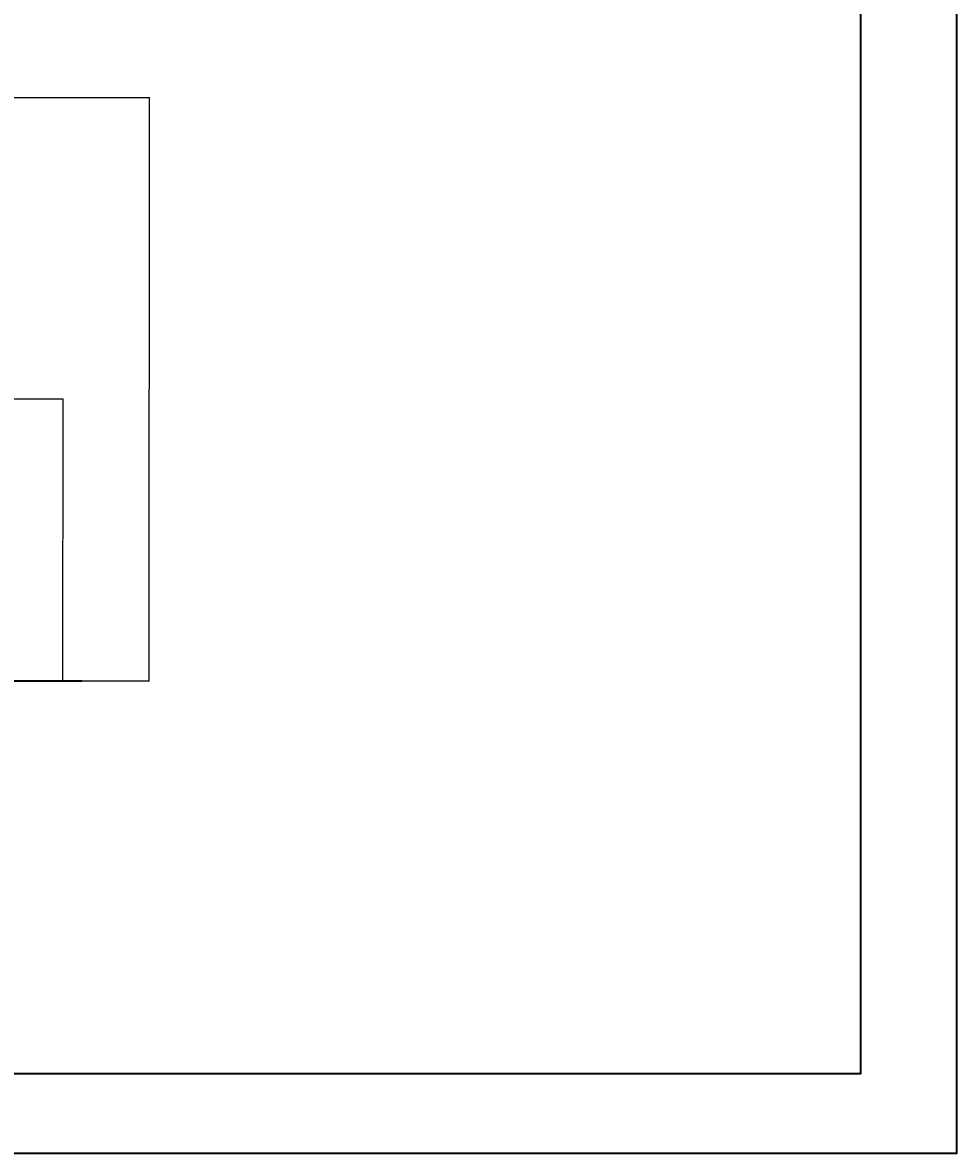
# Model space of a CAD drawing. Units: inches. Extents: x -934 to 898, y -1502 to 444.
# Tile 4 of 10: x 268 to 898, y -1502 to -739. Entities that reach past the tile are written whole.
import ezdxf

# ---------------------------------------------------------------- set-up
doc = ezdxf.new("R2010")
doc.units = ezdxf.units.IN
doc.header["$MEASUREMENT"] = 0
for name, color, linetype, lineweight in [('A-ANNO-DIMS', 2, 'Continuous', 18), ('A-ANNO-TTLB', 7, 'Continuous', 35), ('L-GRND', 7, 'Continuous', 35)]:
    doc.layers.add(name, color=color, linetype=linetype, lineweight=lineweight)
doc.styles.get("Standard").update_dxf_attribs({"font": 'arial.ttf'})
doc.dimstyles.get("Standard").update_dxf_attribs({"dimtxt": 0.18, "dimasz": 0.18, "dimexe": 0.18, "dimexo": 0.0625, "dimgap": 0.09, "dimtad": 0, "dimtih": 1, "dimtoh": 1, "dimdec": 4, "dimzin": 0, "dimdsep": 46, "dimtxsty": 'Standard', "dimcen": 0.09, "dimadec": 0, "dimazin": 0, "dimtfac": 1, "dimtdec": 4, "dimtofl": 0, "dimtmove": 0, "dimatfit": 3, "dimfxl": 1, "dimtolj": 1, "dimtzin": 0, "dimarcsym": 0})

# ---------------------------------------------------------------- blocks, each defined once
blk = doc.blocks.new('*D108')
at = {"layer": 'A-ANNO-DIMS', "color": 0, "lineweight": -2, "transparency": 16777216}
for p, q in [((24.87, -789.83), (353.87, -789.83)), ((353.69, -790.01), (353.69, -986.24)), ((353.69, -1182.83), (353.69, -986.6)), ((250.04, -1183.01), (353.87, -1183.01))]:
    blk.add_line(p, q, dxfattribs=at)
at = {"layer": 'A-ANNO-DIMS', "color": 0, "transparency": 16777216}
for points in [[(353.66, -790.01), (353.72, -790.01), (353.69, -789.83)], [(353.66, -1182.83), (353.72, -1182.83), (353.69, -1183.01)]]:
    blk.add_solid(points, dxfattribs=at)
at = {"layer": 'Defpoints', "color": 0, "transparency": 16777216}
for p in [(24.8, -789.83), (353.69, -789.83), (249.98, -1183.01)]:
    blk.add_point(p, dxfattribs=at)
at = {"layer": 'A-ANNO-DIMS', "color": 0, "transparency": 16777216, "insert": (353.69, -986.42), "char_height": 0.18, "attachment_point": 5}
blk.add_mtext('\\A1;393.2', dxfattribs=at)
blk = doc.blocks.new('*D113')
at = {"layer": 'A-ANNO-DIMS', "color": 0, "lineweight": -2, "transparency": 16777216}
for p, q in [((250.04, -993.04), (295.66, -993.04)), ((295.48, -993.22), (295.48, -1087.84)), ((295.48, -1182.83), (295.48, -1088.21)), ((250.04, -1183.01), (295.66, -1183.01))]:
    blk.add_line(p, q, dxfattribs=at)
at = {"layer": 'A-ANNO-DIMS', "color": 0, "transparency": 16777216}
for points in [[(295.45, -993.22), (295.51, -993.22), (295.48, -993.04)], [(295.45, -1182.83), (295.51, -1182.83), (295.48, -1183.01)]]:
    blk.add_solid(points, dxfattribs=at)
at = {"layer": 'Defpoints', "color": 0, "transparency": 16777216}
for p in [(249.98, -993.04), (249.98, -1183.01), (295.48, -1183.01)]:
    blk.add_point(p, dxfattribs=at)
at = {"layer": 'A-ANNO-DIMS', "color": 0, "transparency": 16777216, "insert": (295.48, -1088.02), "char_height": 0.18, "attachment_point": 5}
blk.add_mtext('\\A1;189.97', dxfattribs=at)

msp = doc.modelspace()

# ---------------------------------------------------------------- linework, layer by layer
at = {"layer": 'A-ANNO-TTLB'}
for points in [[(-933.5092, 444.4646), (897.7239, 444.4646), (897.7239, -1501.5858), (-933.5092, -1501.5858)], [(-892.081, 380.0228), (832.9871, 380.0228), (832.9871, -1448.0237), (-892.081, -1448.0237)]]:
    msp.add_lwpolyline(points, close=True, dxfattribs=at)
at = {"layer": 'L-GRND'}
msp.add_line((-288.9776, -1183.0104), (308.1933, -1183.0104), dxfattribs=at)

# ---------------------------------------------------------------- dimensions: what is measured, and where the dimension line sits
at = {"layer": 'A-ANNO-DIMS'}
for base, p1, p2, angle, override, picture, middle in [((353.6933, -789.826), (249.977, -1183.0104), (24.8027, -789.826), 90, {"dimdec": 1, "dimlfac": 1, "dimrnd": 0, "dimzin": 0, "dimdsep": 46, "dimlunit": 2}, '*D108', (353.6933, -986.4182)), ((295.477, -1183.0104), (249.977, -993.0377), (249.977, -1183.0104), 270, {"dimdec": 2, "dimlfac": 1, "dimrnd": 0, "dimzin": 0, "dimdsep": 46, "dimlunit": 2}, '*D113', (295.477, -1088.024))]:
    dim = msp.add_linear_dim(base=base, p1=p1, p2=p2, angle=angle, dimstyle='Standard', override=override, dxfattribs=at)
    dim.commit()
    dim.dimension.update_dxf_attribs({"geometry": picture, "text_midpoint": middle})

doc.saveas('drawing.dxf')
